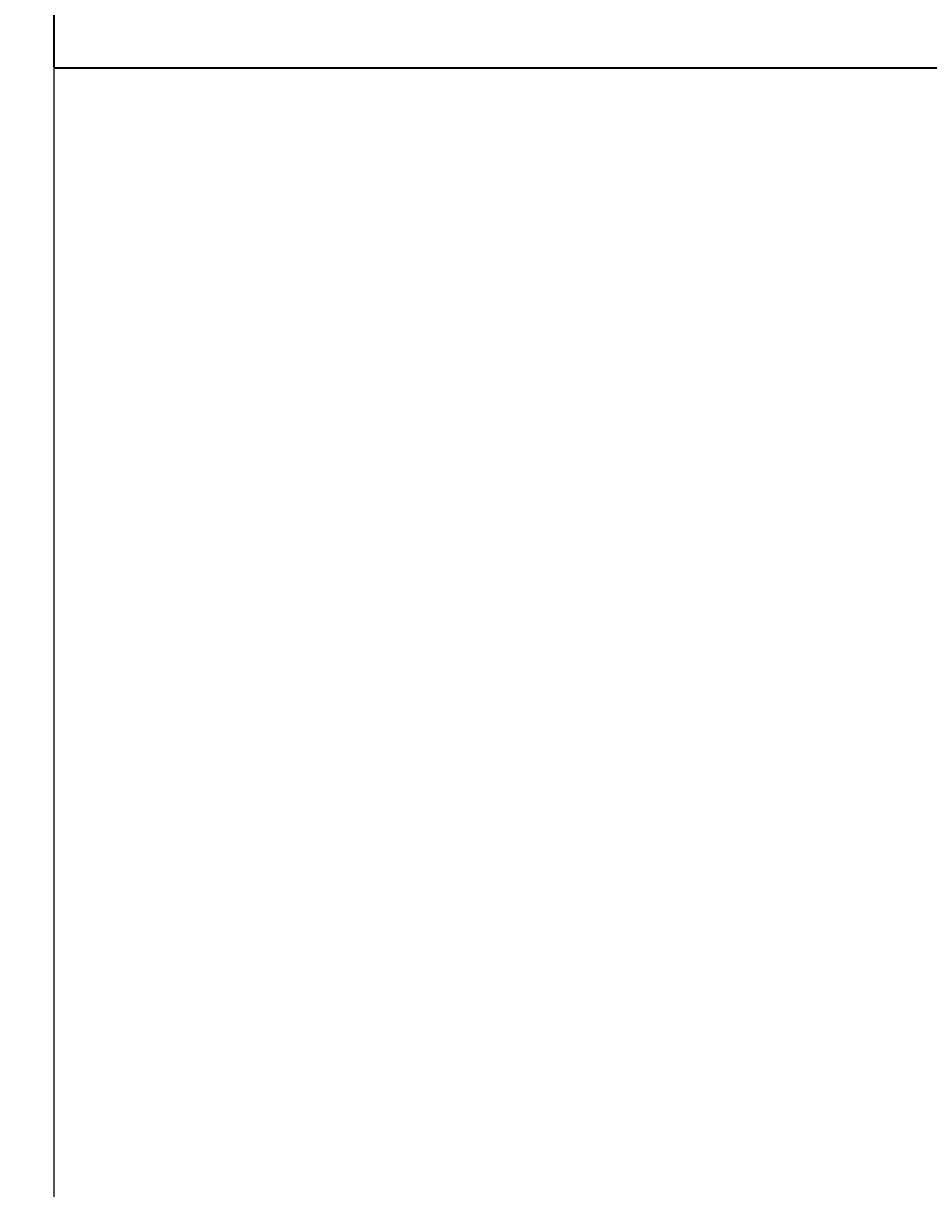
# Model space of a CAD drawing. Units: millimetres. Extents: x 27017497 to 27018854, y 7058029 to 7059154.
# Tile 14 of 91: x 27017560 to 27017605, y 7058238 to 7058297. Entities that reach past the tile are written whole.
import ezdxf

# ---------------------------------------------------------------- set-up
doc = ezdxf.new("R2010")
doc.units = ezdxf.units.MM
doc.layers.add('A-ANNO-DIMS', color=2, linetype='Continuous', lineweight=18)
doc.layers.add('A-WALL', color=7, linetype='Continuous', lineweight=35)
doc.styles.get("Standard").update_dxf_attribs({"font": 'arial.ttf'})
doc.dimstyles.get("Standard").update_dxf_attribs({"dimtxt": 0.18, "dimasz": 0.18, "dimexe": 0.18, "dimexo": 0.0625, "dimgap": 0.09, "dimtad": 0, "dimtih": 1, "dimtoh": 1, "dimdec": 4, "dimzin": 0, "dimdsep": 46, "dimtxsty": 'Standard', "dimcen": 0.09, "dimadec": 0, "dimazin": 0, "dimtfac": 1, "dimtdec": 4, "dimtofl": 0, "dimtmove": 0, "dimatfit": 3, "dimfxl": 1, "dimtolj": 1, "dimtzin": 0, "dimarcsym": 0})

# ---------------------------------------------------------------- blocks, each defined once
blk = doc.blocks.new('*D47')
at = {"layer": 'A-ANNO-DIMS', "color": 0, "lineweight": -2, "transparency": 16777216}
for p, q in [((27017561.166, 7058294.35), (27017561.166, 7058028.6)), ((27018790.606, 7058294.35), (27018790.606, 7058028.6)), ((27017561.346, 7058028.78), (27018175.431, 7058028.78)), ((27018790.426, 7058028.78), (27018176.341, 7058028.78))]:
    blk.add_line(p, q, dxfattribs=at)
at = {"layer": 'A-ANNO-DIMS', "color": 0, "transparency": 16777216}
for points in [[(27017561.346, 7058028.81), (27017561.346, 7058028.75), (27017561.166, 7058028.78)], [(27018790.426, 7058028.81), (27018790.426, 7058028.75), (27018790.606, 7058028.78)]]:
    blk.add_solid(points, dxfattribs=at)
at = {"layer": 'Defpoints', "color": 0, "transparency": 16777216}
for p in [(27017561.166, 7058294.412), (27018790.606, 7058294.412), (27018790.606, 7058028.78)]:
    blk.add_point(p, dxfattribs=at)
at = {"layer": 'A-ANNO-DIMS', "color": 0, "transparency": 16777216, "insert": (27018175.886, 7058028.78), "char_height": 0.18, "attachment_point": 5}
blk.add_mtext('\\A1;1229.4', dxfattribs=at)
blk = doc.blocks.new('*D48')
at = {"layer": 'A-ANNO-DIMS', "color": 0, "lineweight": -2, "transparency": 16777216}
for p, q in [((27018463.498, 7058622.912), (27017497.536, 7058622.912)), ((27017497.716, 7058622.732), (27017497.716, 7058357.753)), ((27017497.716, 7058092.41), (27017497.716, 7058357.389)), ((27018555.129, 7058092.23), (27017497.536, 7058092.23))]:
    blk.add_line(p, q, dxfattribs=at)
at = {"layer": 'A-ANNO-DIMS', "color": 0, "transparency": 16777216}
for points in [[(27017497.686, 7058622.732), (27017497.746, 7058622.732), (27017497.716, 7058622.912)], [(27017497.686, 7058092.41), (27017497.746, 7058092.41), (27017497.716, 7058092.23)]]:
    blk.add_solid(points, dxfattribs=at)
at = {"layer": 'Defpoints', "color": 0, "transparency": 16777216}
for p in [(27018463.561, 7058622.912), (27017497.716, 7058092.23), (27018555.192, 7058092.23)]:
    blk.add_point(p, dxfattribs=at)
at = {"layer": 'A-ANNO-DIMS', "color": 0, "transparency": 16777216, "insert": (27017497.716, 7058357.571), "char_height": 0.18, "attachment_point": 5}
blk.add_mtext('\\A1;530.7', dxfattribs=at)

msp = doc.modelspace()

# ---------------------------------------------------------------- linework, layer by layer
at = {"layer": 'A-WALL'}
for p, q in [((27017561.166, 7058437.098), (27017561.166, 7058294.412)), ((27017561.166, 7058294.412), (27017613.666, 7058294.412))]:
    msp.add_line(p, q, dxfattribs=at)

# ---------------------------------------------------------------- dimensions: what is measured, and where the dimension line sits
at = {"layer": 'A-ANNO-DIMS'}
dim = msp.add_linear_dim(base=(27017497.716, 7058092.23), p1=(27018463.561, 7058622.912), p2=(27018555.192, 7058092.23), angle=90, dimstyle='Standard', override={"dimdec": 1, "dimlfac": 1, "dimrnd": 0, "dimzin": 0, "dimdsep": 46, "dimlunit": 2}, dxfattribs=at)
dim.commit()
dim.dimension.update_dxf_attribs({"geometry": '*D48', "text_midpoint": (27017497.716, 7058357.571)})
dim = msp.add_linear_dim(base=(27018790.606, 7058028.78), p1=(27017561.166, 7058294.412), p2=(27018790.606, 7058294.412), dimstyle='Standard', override={"dimdec": 1, "dimlfac": 1, "dimrnd": 0, "dimzin": 0, "dimdsep": 46, "dimlunit": 2}, dxfattribs=at)
dim.commit()
dim.dimension.update_dxf_attribs({"geometry": '*D47', "text_midpoint": (27018175.886, 7058028.78)})

doc.saveas('drawing.dxf')
